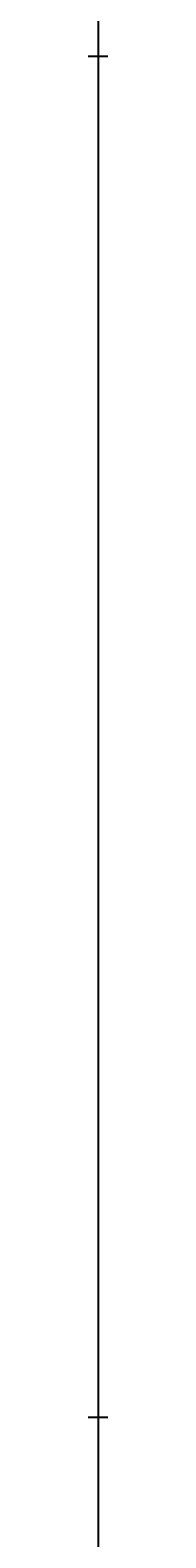
# Model space of a CAD drawing. Units: inches. Extents: x 35362 to 73946, y 43607 to 67532.
# Tile 26 of 134: x 48373 to 48373, y 46091 to 46564. Entities that reach past the tile are written whole.
import ezdxf

# ---------------------------------------------------------------- set-up
doc = ezdxf.new("R2010")
doc.units = ezdxf.units.IN
doc.header["$MEASUREMENT"] = 0
doc.layers.add('A-ANNO-DIMS', color=2, linetype='Continuous', lineweight=18)
doc.styles.get("Standard").update_dxf_attribs({"font": 'arial.ttf'})
doc.dimstyles.get("Standard").update_dxf_attribs({"dimtxt": 0.18, "dimasz": 0.18, "dimexe": 0.18, "dimexo": 0.0625, "dimgap": 0.09, "dimtad": 0, "dimtih": 1, "dimtoh": 1, "dimdec": 4, "dimzin": 0, "dimdsep": 46, "dimtxsty": 'Standard', "dimcen": 0.09, "dimadec": 0, "dimazin": 0, "dimtfac": 1, "dimtdec": 4, "dimtofl": 0, "dimtmove": 0, "dimatfit": 3, "dimfxl": 1, "dimtolj": 1, "dimtzin": 0, "dimarcsym": 0})

# ---------------------------------------------------------------- blocks, each defined once
blk = doc.blocks.new('*D5')
at = {"layer": 'A-ANNO-DIMS', "color": 0, "lineweight": -2, "transparency": 16777216}
for p, q in [((37121.95, 46919.32), (37121.95, 43606.68)), ((69871.5, 45449.83), (69871.5, 43606.68)), ((37122.13, 43606.86), (53496.29, 43606.86)), ((69871.32, 43606.86), (53497.15, 43606.86))]:
    blk.add_line(p, q, dxfattribs=at)
at = {"layer": 'A-ANNO-DIMS', "color": 0, "transparency": 16777216}
for points in [[(37122.13, 43606.89), (37122.13, 43606.83), (37121.95, 43606.86)], [(69871.32, 43606.89), (69871.32, 43606.83), (69871.5, 43606.86)]]:
    blk.add_solid(points, dxfattribs=at)
at = {"layer": 'Defpoints', "color": 0, "transparency": 16777216}
for p in [(37121.95, 46919.38), (69871.5, 45449.89), (69871.5, 43606.86)]:
    blk.add_point(p, dxfattribs=at)
at = {"layer": 'A-ANNO-DIMS', "color": 0, "transparency": 16777216, "insert": (53496.72, 43606.86), "char_height": 0.18, "attachment_point": 5}
blk.add_mtext('\\A1;32750', dxfattribs=at)
blk = doc.blocks.new('*D11')
at = {"layer": 'A-ANNO-DIMS', "color": 0, "lineweight": -2, "transparency": 16777216}
for p, q in [((47978.66, 56028.77), (47978.66, 43606.68)), ((53109.76, 56028.77), (53109.76, 43606.68)), ((47978.84, 43606.86), (50543.87, 43606.86)), ((53109.58, 43606.86), (50544.55, 43606.86))]:
    blk.add_line(p, q, dxfattribs=at)
at = {"layer": 'A-ANNO-DIMS', "color": 0, "transparency": 16777216}
for points in [[(47978.84, 43606.89), (47978.84, 43606.83), (47978.66, 43606.86)], [(53109.58, 43606.89), (53109.58, 43606.83), (53109.76, 43606.86)]]:
    blk.add_solid(points, dxfattribs=at)
at = {"layer": 'Defpoints', "color": 0, "transparency": 16777216}
for p in [(47978.66, 56028.84), (53109.76, 56028.84), (53109.76, 43606.86)]:
    blk.add_point(p, dxfattribs=at)
at = {"layer": 'A-ANNO-DIMS', "color": 0, "transparency": 16777216, "insert": (50544.21, 43606.86), "char_height": 0.18, "attachment_point": 5}
blk.add_mtext('\\A1;5131', dxfattribs=at)
blk = doc.blocks.new('*D27')
at = {"layer": 'A-ANNO-DIMS', "color": 0, "lineweight": -2, "transparency": 16777216}
for p, q in [((47978.66, 56028.77), (47978.66, 43606.68)), ((48373.49, 53428.96), (48373.49, 43606.68)), ((47978.84, 43606.86), (48175.68, 43606.86)), ((48373.31, 43606.86), (48176.47, 43606.86))]:
    blk.add_line(p, q, dxfattribs=at)
at = {"layer": 'A-ANNO-DIMS', "color": 0, "transparency": 16777216}
for points in [[(47978.84, 43606.89), (47978.84, 43606.83), (47978.66, 43606.86)], [(48373.31, 43606.89), (48373.31, 43606.83), (48373.49, 43606.86)]]:
    blk.add_solid(points, dxfattribs=at)
at = {"layer": 'Defpoints', "color": 0, "transparency": 16777216}
for p in [(47978.66, 56028.84), (48373.49, 53429.02), (48373.49, 43606.86)]:
    blk.add_point(p, dxfattribs=at)
at = {"layer": 'A-ANNO-DIMS', "color": 0, "transparency": 16777216, "insert": (48176.08, 43606.86), "char_height": 0.18, "attachment_point": 5}
blk.add_mtext('\\A1;394.8', dxfattribs=at)
blk = doc.blocks.new('*D67')
at = {"layer": 'A-ANNO-DIMS', "color": 0, "lineweight": -2, "transparency": 16777216}
for p, q in [((56873.54, 53351.53), (35361.77, 53351.53)), ((35361.95, 53351.35), (35361.95, 49400.89)), ((35361.95, 45450.07), (35361.95, 49400.53)), ((53793.58, 45449.89), (35361.77, 45449.89))]:
    blk.add_line(p, q, dxfattribs=at)
at = {"layer": 'A-ANNO-DIMS', "color": 0, "transparency": 16777216}
for points in [[(35361.92, 53351.35), (35361.98, 53351.35), (35361.95, 53351.53)], [(35361.92, 45450.07), (35361.98, 45450.07), (35361.95, 45449.89)]]:
    blk.add_solid(points, dxfattribs=at)
at = {"layer": 'Defpoints', "color": 0, "transparency": 16777216}
for p in [(35361.95, 53351.53), (56873.6, 53351.53), (53793.64, 45449.89)]:
    blk.add_point(p, dxfattribs=at)
at = {"layer": 'A-ANNO-DIMS', "color": 0, "transparency": 16777216, "insert": (35361.95, 49400.71), "char_height": 0.18, "attachment_point": 5}
blk.add_mtext('\\A1;7901.6', dxfattribs=at)
blk = doc.blocks.new('*D76')
at = {"layer": 'A-ANNO-DIMS', "color": 0, "lineweight": -2, "transparency": 16777216}
for p, q in [((54052.84, 46555.29), (35361.77, 46555.29)), ((35361.95, 46555.11), (35361.95, 46342.27)), ((35361.95, 46129.06), (35361.95, 46341.9)), ((53793.58, 46128.88), (35361.77, 46128.88))]:
    blk.add_line(p, q, dxfattribs=at)
at = {"layer": 'A-ANNO-DIMS', "color": 0, "transparency": 16777216}
for points in [[(35361.92, 46555.11), (35361.98, 46555.11), (35361.95, 46555.29)], [(35361.92, 46129.06), (35361.98, 46129.06), (35361.95, 46128.88)]]:
    blk.add_solid(points, dxfattribs=at)
at = {"layer": 'Defpoints', "color": 0, "transparency": 16777216}
for p in [(35361.95, 46555.29), (54052.9, 46555.29), (53793.64, 46128.88)]:
    blk.add_point(p, dxfattribs=at)
at = {"layer": 'A-ANNO-DIMS', "color": 0, "transparency": 16777216, "insert": (35361.95, 46342.09), "char_height": 0.18, "attachment_point": 5}
blk.add_mtext('\\A1;426.4', dxfattribs=at)
blk = doc.blocks.new('*D90')
at = {"layer": 'A-ANNO-DIMS', "color": 0, "lineweight": -2, "transparency": 16777216}
for p, q in [((53707.72, 47291.29), (35361.77, 47291.29)), ((35361.95, 47291.11), (35361.95, 46710.26)), ((35361.95, 46129.06), (35361.95, 46709.9)), ((53793.58, 46128.88), (35361.77, 46128.88))]:
    blk.add_line(p, q, dxfattribs=at)
at = {"layer": 'A-ANNO-DIMS', "color": 0, "transparency": 16777216}
for points in [[(35361.92, 47291.11), (35361.98, 47291.11), (35361.95, 47291.29)], [(35361.92, 46129.06), (35361.98, 46129.06), (35361.95, 46128.88)]]:
    blk.add_solid(points, dxfattribs=at)
at = {"layer": 'Defpoints', "color": 0, "transparency": 16777216}
for p in [(53707.78, 47291.29), (35361.95, 46128.88), (53793.64, 46128.88)]:
    blk.add_point(p, dxfattribs=at)
at = {"layer": 'A-ANNO-DIMS', "color": 0, "transparency": 16777216, "insert": (35361.95, 46710.08), "char_height": 0.18, "attachment_point": 5}
blk.add_mtext('\\A1;1162.4', dxfattribs=at)

msp = doc.modelspace()

# ---------------------------------------------------------------- dimensions: what is measured, and where the dimension line sits
at = {"layer": 'A-ANNO-DIMS'}
for base, p1, p2, override, picture, middle in [((53109.76, 43606.859), (47978.665, 56028.836), (53109.76, 56028.836), {"dimdec": 0, "dimlfac": 1, "dimrnd": 0, "dimzin": 0, "dimdsep": 46, "dimlunit": 2}, '*D11', (50544.212, 43606.859)), ((48373.492, 43606.859), (47978.665, 56028.836), (48373.492, 53429.019), {"dimdec": 1, "dimlfac": 1, "dimrnd": 0, "dimzin": 0, "dimdsep": 46, "dimlunit": 2}, '*D27', (48176.078, 43606.859)), ((69871.496, 43606.859), (37121.949, 46919.381), (69871.496, 45449.894), {"dimdec": 0, "dimlfac": 1, "dimrnd": 0, "dimzin": 0, "dimdsep": 46, "dimlunit": 2}, '*D5', (53496.723, 43606.859))]:
    dim = msp.add_linear_dim(base=base, p1=p1, p2=p2, dimstyle='Standard', override=override, dxfattribs=at)
    dim.commit()
    dim.dimension.update_dxf_attribs({"geometry": picture, "text_midpoint": middle})
for base, p1, p2, picture, middle in [((35361.949, 53351.529), (53793.638, 45449.894), (56873.602, 53351.529), '*D67', (35361.949, 49400.712)), ((35361.949, 46128.878), (53707.781, 47291.285), (53793.638, 46128.878), '*D90', (35361.949, 46710.081)), ((35361.949, 46555.293), (53793.638, 46128.878), (54052.899, 46555.293), '*D76', (35361.949, 46342.086))]:
    dim = msp.add_linear_dim(base=base, p1=p1, p2=p2, angle=90, dimstyle='Standard', override={"dimdec": 1, "dimlfac": 1, "dimrnd": 0, "dimzin": 0, "dimdsep": 46, "dimlunit": 2}, dxfattribs=at)
    dim.commit()
    dim.dimension.update_dxf_attribs({"geometry": picture, "text_midpoint": middle})

doc.saveas('drawing.dxf')
